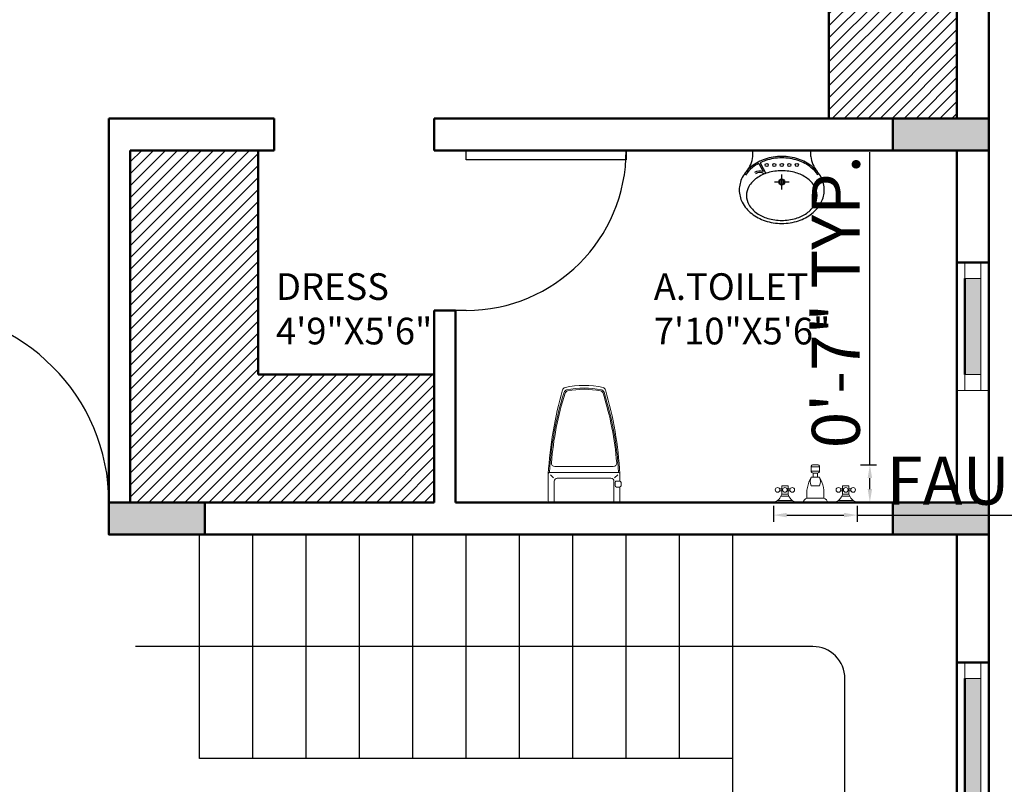
# Model space of a CAD drawing. Units: inches. Extents: x 3064 to 19385, y 846 to 15425.
# Tile 19 of 108: x 3808 to 3992, y 1134 to 1277. Entities that reach past the tile are written whole.
import ezdxf

# ---------------------------------------------------------------- set-up
doc = ezdxf.new("R2010")
doc.units = ezdxf.units.IN
for name, color, linetype, lineweight in [('A-ANNO-DIMS', 2, 'Continuous', 18), ('A-AREA-IDEN', 3, 'Continuous', 18), ('A-COLS', 1, 'Continuous', 35), ('A-DOOR', 3, 'Continuous', 25), ('A-FLOR-FIXT', 9, 'Continuous', 18), ('A-FLOR-STRS', 2, 'Continuous', 25), ('A-FURN-PATT', 252, 'Continuous', 13), ('A-GLAZ', 4, 'Continuous', 18), ('A-WALL', 7, 'Continuous', 50)]:
    doc.layers.add(name, color=color, linetype=linetype, lineweight=lineweight)
doc.layers.add('THIET-BI', color=21, linetype='Continuous')
doc.styles.get("Standard").update_dxf_attribs({"font": 'arial.ttf'})
doc.dimstyles.new('ISO-25', dxfattribs={"dimtxt": 9, "dimasz": 2.5, "dimexe": 1.25, "dimexo": 0.625, "dimtad": 1, "dimdec": 1, "dimlunit": 3, "dimtxsty": 'Standard', "dimcen": 2.5, "dimadec": 0, "dimazin": 0, "dimtfac": 1, "dimtdec": 1, "dimtmove": 0, "dimatfit": 3, "dimfxl": 1, "dimarcsym": 0})
pattern_1 = [(45, (-695.1336, 0), (-1.122532, 1.122532), [])]

# ---------------------------------------------------------------- blocks, each defined once
blk = doc.blocks.new('*U3')
for p, q in [((0, 0), (0, -6)), ((36, 0), (36, -6))]:
    blk.add_line(p, q)
blk.add_lwpolyline([(0, 0), (0, 36), (1.75, 36), (1.75, 0)], close=True)
blk.add_arc((0, 0), 36, 0, 90)
blk = doc.blocks.new('*U4')
for p, q in [((0, 0), (0, -6)), ((30, 0), (30, -6))]:
    blk.add_line(p, q)
blk.add_lwpolyline([(0, 0), (0, 30), (1.75, 30), (1.75, 0)], close=True)
blk.add_arc((0, 0), 30, 0, 90)
blk = doc.blocks.new('A$C430D11A0')
at = {"layer": 'THIET-BI'}
for p, q in [((90, 445), (90, 485)), ((475, 485), (90, 485)), ((475, 483), (90, 483)), ((475, 445), (475, 485)), ((129.4, 398.5), (158.2, 344.4)), ((138.3, 403), (176, 332.4)), ((233.4, 275.5), (331.9, 275.5)), ((282.5, 226.2), (282.5, 324.8))]:
    blk.add_line(p, q, dxfattribs=at)
for points in [[(565, 222.5, 0.121635), (544.7, 304.8, 0.10526), (482.3, 379.8, 0.088175), (393.4, 427.4, 0.079002), (282.5, 445, 0.079002), (171.6, 427.4, 0.088175), (82.7, 379.8, 0.10526), (20.3, 304.8, 0.121635), (0, 222.5, 0.121635), (20.3, 140.2, 0.10526), (82.7, 65.2, 0.088175), (171.6, 17.6, 0.079002), (282.5, 0, 0.079002), (393.4, 17.6, 0.088175), (482.3, 65.2, 0.10526), (544.7, 140.2, 0.121635)], [(517.5, 185, 0.134042), (501.2, 244.9, 0.106817), (448.7, 301.7, 0.082468), (375.6, 336.7, 0.070874), (282.5, 350, 0.070874), (189.4, 336.7, 0.082468), (116.3, 301.7, 0.106817), (63.8, 244.9, 0.134042), (47.5, 185, 0.134042), (63.8, 125.1, 0.106817), (116.3, 68.3, 0.082468), (189.4, 33.3, 0.070874), (282.5, 20, 0.070874), (375.6, 33.3, 0.082468), (448.7, 68.3, 0.106817), (501.2, 125.1, 0.134042)]]:
    blk.add_lwpolyline(points, format="xyb", close=True, dxfattribs=at)
for points in [[(129.4, 398.5, 0.043566), (88.9, 372, 0.07708), (42.1, 321.6, 0.041486)], [(522.9, 321.6, 0.07708), (476.1, 372, 0.088175), (390.3, 417.9, 0.079002), (282.5, 435, 0.079002), (174.7, 417.9, 0.035427), (138.3, 403, 0.07708)]]:
    blk.add_lwpolyline(points, format="xyb", dxfattribs=at)
for centre, radius in [((182.5, 388.2), 10.5), ((232.5, 388.2), 10.5), ((282.5, 388.2), 10.5), ((332.5, 388.2), 10.5), ((382.5, 388.2), 10.5), ((282.5, 275.5), 20), ((282.5, 275.5), 15)]:
    blk.add_circle(centre, radius, dxfattribs=at)
for centre, radius, start, end in [((-103.8, 468.9), 195.3, 320.8253, 352.95569), ((668.8, 468.9), 195.3, 187.04431, 219.1747), ((136.4, 285.4), 62.9, 69.64296, 123.47738), ((136.4, 285.4), 52.9, 55.24551, 123.47738)]:
    blk.add_arc(centre, radius, start, end, dxfattribs=at)
blk = doc.blocks.new('WC-P05')
for p, q in [((-202.4, 531.6), (-202.4, 439.1)), ((-192.4, 541.6), (262.6, 541.6)), ((-163.4, 541.6), (-163.4, 400.6)), ((233.6, 541.6), (233.6, 400.6)), ((272.6, 531.6), (272.6, 351.6)), ((-210.4, 430.1), (-210.4, 409.1)), ((-202.4, 400.1), (-202.4, 351.6)), ((-201.4, 439.1), (-180.4, 439.1)), ((-201.4, 400.1), (-180.4, 400.1)), ((-171.4, 430.1), (-171.4, 409.1)), ((-192.4, 341.6), (262.6, 341.6)), ((-166.9, 378.6), (-188.2, 357.3)), ((-143.4, 380.6), (213.6, 380.6)), ((237.1, 378.6), (258.4, 357.3)), ((-159.3, 302.6), (229.5, 302.6))]:
    blk.add_line(p, q)
blk.add_lwpolyline([(-90.9, -221.9, 0.114547), (161, -222, 0.114547)], format="xyb")
for centre, radius, start, end in [((-192.4, 531.6), 10, 90, 180), ((262.6, 531.6), 10, 0, 90), ((-201.4, 430.1), 9, 90, 180), ((-201.4, 409.1), 9, 180, 270), ((-180.4, 430.1), 9, 0, 90), ((-180.4, 409.1), 9, 270, 0), ((-143.4, 400.6), 20, 180, 270), ((213.6, 400.6), 20, 270, 0), ((2308.9, 492.3), 2515.2, 183.20675, 196.12415), ((-192.4, 351.6), 10, 180, 270), ((1906, 447.2), 2102.6, 182.87428, 197.65536), ((-1835.8, 447.2), 2102.6, 342.34464, 357.12572), ((-2238.7, 492.3), 2515.2, 343.87268, 356.79325), ((262.6, 351.6), 10, 270, 0), ((-159.3, 280.1), 22.5, 90, 184.62462), ((1905.9, 447.2), 2094.5, 184.62454, 197.52765), ((-1835.8, 447.2), 2094.6, 342.46396, 355.37538), ((229.5, 280.1), 22.5, 355.37538, 90), ((-76.1, -183.7), 22.5, 197.65536, 257.50587), ((-69.9, -176.8), 22.5, 197.52765, 258.10049), ((139.9, -177.1), 22.5, 281.73735, 342.46396), ((146.2, -183.7), 22.5, 282.49413, 342.34464), ((-85.8, -199.9), 22.5, 196.12415, 256.89941), ((35.1, 318), 536.4, 257.50587, 282.49413), ((35.7, 324.3), 534.7, 258.10049, 281.73735), ((155.9, -200.1), 22.5, 283.03778, 343.87268)]:
    blk.add_arc(centre, radius, start, end)
blk = doc.blocks.new('Faucet - Bathroom front')
for p, q in [((-0.5, 4.25), (0.5, 4.25)), ((0.5, 3.75), (-0.5, 3.75)), ((-0.5, 3), (0.5, 3)), ((-0.25, 3), (-0.25, 3.5)), ((0.25, 3.5), (0.25, 3)), ((-4, 1.625), (-4.25, 1.625)), ((-4, 1.375), (-4.25, 1.375)), ((-3.25, 1.625), (-3, 1.625)), ((-3.25, 1.375), (-3, 1.375)), ((0.5, 2), (-0.5, 2)), ((3.25, 1.625), (3, 1.625)), ((3.25, 1.375), (3, 1.375)), ((4, 1.625), (4.25, 1.625)), ((4, 1.375), (4.25, 1.375)), ((-5, 0), (-2.25, 0)), ((-4.5087, 0.25), (-2.7408, 0.25)), ((-3.1442, 0.75), (-4.0979, 0.75)), ((-1.5, 0), (1.5, 0)), ((-1, 0.5), (1, 0.5)), ((2.25, 0), (5, 0)), ((2.7413, 0.25), (4.5092, 0.25)), ((4.1058, 0.75), (3.1521, 0.75))]:
    blk.add_line(p, q)
for points in [[(-0.5, 3.75), (-0.5, 4.25)], [(-0.25, 4.5), (0.25, 4.5)], [(0.5, 4.25), (0.5, 3.75)], [(0.25, 3.5), (-0.25, 3.5)]]:
    blk.add_lwpolyline(points)
for points in [[(-4, 1), (-4, 2), (-3.25, 2), (-3.25, 1)], [(3.25, 1), (3.25, 2), (4, 2), (4, 1)]]:
    blk.add_lwpolyline(points, close=True)
for centre in [(-4.5, 1.5), (-3.625, 1.5), (-2.75, 1.5), (2.75, 1.5), (3.625, 1.5), (4.5, 1.5)]:
    blk.add_circle(centre, 0.2795)
for centre, radius, start, end in [((-0.2575, 4.2575), 0.2426, 88.22243, 181.7776), ((-0.2575, 3.7425), 0.2426, 178.2224, 271.7776), ((0.2575, 4.2575), 0.2426, 358.2224, 91.77757), ((0.2575, 3.7425), 0.2426, 268.2224, 1.777565), ((3, 1), 4.0311, 150.2551, 187.125), ((0.6413, 2.5), 1.246, 156.3417, 203.6583), ((-3, 1), 4.0311, 352.875, 29.74488), ((-0.6413, 2.5), 1.246, 336.3417, 23.65835), ((-5.375, 1.375), 1.4252, 285.2551, 344.7449), ((-1.875, 1.375), 1.4252, 195.2551, 254.7449), ((-0.7962, -0.2038), 0.7327, 106.1502, 163.8498), ((0.7962, -0.2038), 0.7327, 16.1502, 73.84979), ((1.875, 1.375), 1.4252, 285.2551, 344.7449), ((5.375, 1.375), 1.4252, 195.2551, 254.7449)]:
    blk.add_arc(centre, radius, start, end)
blk = doc.blocks.new('WIN-600')
h = blk.add_hatch(color=256)
h.dxf.hatch_style = 1
h.paths.add_polyline_path([(3, 18), (0, 18), (0, 0), (3, 0)])
blk.add_line((3, 18), (3, 0))
blk.add_lwpolyline([(3, 18), (0, 18), (0, 21), (3, 21)], close=True)
blk = doc.blocks.new('WIN-1800-PAIR')
h = blk.add_hatch(color=256)
h.dxf.hatch_style = 1
h.paths.add_polyline_path([(0, 0), (3, 0), (3, 70.5), (0, 70.5)])
h.paths.add_polyline_path([(3, 144), (0, 144), (0, 73.5), (3, 73.5)])
blk.add_line((3, 144), (3, 73.5))
blk.add_lwpolyline([(3, 144), (0, 144), (0, 147), (3, 147)], close=True)
blk = doc.blocks.new('*D407')
at = {"layer": 'A-ANNO-DIMS', "color": 0, "lineweight": -2, "transparency": 16777216}
for p, q in [((3948.96, 1185.71), (3948.96, 1182.73)), ((3964.69, 1185.71), (3964.69, 1182.73)), ((3951.46, 1183.98), (3962.19, 1183.98)), ((3964.69, 1183.98), (4097.55, 1183.98))]:
    blk.add_line(p, q, dxfattribs=at)
at = {"layer": 'A-ANNO-DIMS', "color": 0, "transparency": 16777216}
for points in [[(3951.46, 1184.4), (3951.46, 1183.56), (3948.96, 1183.98)], [(3962.19, 1184.4), (3962.19, 1183.56), (3964.69, 1183.98)]]:
    blk.add_solid(points, dxfattribs=at)
at = {"layer": 'Defpoints', "color": 0, "transparency": 16777216}
for p in [(3948.96, 1186.34), (3964.69, 1186.34), (3964.69, 1183.98)]:
    blk.add_point(p, dxfattribs=at)
at = {"layer": 'A-ANNO-DIMS', "color": 0, "transparency": 16777216, "insert": (4032.37, 1189.26), "char_height": 9, "attachment_point": 5}
blk.add_mtext('FAUCET 1\'-3 1/2" TYP.', dxfattribs=at)
blk = doc.blocks.new('*D408')
at = {"layer": 'A-ANNO-DIMS', "color": 0, "lineweight": -2, "transparency": 16777216}
for p, q in [((3967.05, 1193.42), (3967.05, 1252.03)), ((3965.32, 1193.42), (3968.3, 1193.42)), ((3967.05, 1188.84), (3967.05, 1190.92)), ((3965.32, 1186.34), (3968.3, 1186.34))]:
    blk.add_line(p, q, dxfattribs=at)
at = {"layer": 'A-ANNO-DIMS', "color": 0, "transparency": 16777216}
for points in [[(3966.64, 1190.92), (3967.47, 1190.92), (3967.05, 1193.42)], [(3966.64, 1188.84), (3967.47, 1188.84), (3967.05, 1186.34)]]:
    blk.add_solid(points, dxfattribs=at)
at = {"layer": 'Defpoints', "color": 0, "transparency": 16777216}
for p in [(3964.69, 1193.42), (3967.05, 1193.42), (3964.69, 1186.34)]:
    blk.add_point(p, dxfattribs=at)
at = {"layer": 'A-ANNO-DIMS', "color": 0, "transparency": 16777216, "insert": (3961.83, 1223.98), "char_height": 9, "attachment_point": 5, "rotation": 90}
blk.add_mtext('0\'-7" TYP.', dxfattribs=at)

msp = doc.modelspace()

# ---------------------------------------------------------------- hatches: boundary and pattern name
at = {"layer": 'A-COLS'}
h = msp.add_hatch(color=256, dxfattribs=at)
h.dxf.hatch_style = 1
h.paths.add_polyline_path([(3989.36, 1252.34), (3989.36, 1258.34), (3971.36, 1258.34), (3971.36, 1252.34)])
h = msp.add_hatch(color=256, dxfattribs=at)
h.dxf.hatch_style = 1
h.paths.add_polyline_path([(3842.36, 1180.34), (3842.36, 1186.34), (3824.36, 1186.34), (3824.36, 1180.34)])
h = msp.add_hatch(color=256, dxfattribs=at)
h.dxf.hatch_style = 1
h.paths.add_polyline_path([(3989.36, 1180.34), (3989.36, 1186.34), (3971.36, 1186.34), (3971.36, 1180.34)])
at = {"layer": 'A-FURN-PATT'}
h = msp.add_hatch(dxfattribs=at)
h.set_pattern_fill('ANSI31', color=256, scale=0.5)
h.set_pattern_definition(pattern_1)
h.paths.add_polyline_path([(3959.36, 1258.34), (3983.36, 1258.34), (3983.36, 1390.34), (3959.36, 1390.34)])
h = msp.add_hatch(dxfattribs=at)
h.set_pattern_fill('ANSI31', color=256, scale=0.5)
h.set_pattern_definition(pattern_1)
h.paths.add_polyline_path([(3852.36, 1210.34), (3852.36, 1252.34), (3828.36, 1252.34), (3828.36, 1186.34), (3842.36, 1186.34), (3885.36, 1186.34), (3885.36, 1210.34)])

# ---------------------------------------------------------------- linework, layer by layer
at = {"layer": 'A-FLOR-STRS'}
for p, q in [((3841.36, 1138.34), (3841.36, 1180.34)), ((3851.36, 1138.34), (3851.36, 1180.34)), ((3861.36, 1138.34), (3861.36, 1180.34)), ((3871.36, 1138.34), (3871.36, 1180.34)), ((3881.36, 1138.34), (3881.36, 1180.34)), ((3891.36, 1138.34), (3891.36, 1180.34)), ((3901.36, 1138.34), (3901.36, 1180.34)), ((3911.36, 1138.34), (3911.36, 1180.34)), ((3921.36, 1138.34), (3921.36, 1180.34)), ((3931.36, 1138.34), (3931.36, 1180.34)), ((3941.36, 1024.34), (3941.36, 1180.34)), ((3941.36, 1138.34), (3841.36, 1138.34))]:
    msp.add_line(p, q, dxfattribs=at)
msp.add_lwpolyline([(3848.85, 1003.34), (3956.36, 1003.34, 0.414214), (3962.36, 1009.34), (3962.36, 1153.34, 0.414214), (3956.36, 1159.34), (3829.36, 1159.34)], format="xyb", dxfattribs=at)
at = {"layer": 'A-GLAZ'}
msp.add_line((3983.36, 1207.34), (3989.36, 1207.34), dxfattribs=at)
msp.add_lwpolyline([(3987.86, 1207.34), (3984.86, 1207.34), (3984.86, 1210.34), (3987.86, 1210.34)], close=True, dxfattribs=at)
at = {"layer": 'A-WALL'}
for p, q in [((3989.36, 904.34), (3989.36, 1396.34)), ((3959.36, 1258.34), (3959.36, 1390.34)), ((3983.36, 1258.34), (3983.36, 1390.34)), ((3824.36, 1258.34), (3824.36, 1180.34)), ((3855.36, 1258.34), (3824.36, 1258.34)), ((3855.36, 1258.34), (3855.36, 1252.34)), ((3983.36, 1258.34), (3885.36, 1258.34)), ((3885.36, 1258.34), (3885.36, 1252.34)), ((3855.36, 1252.34), (3828.36, 1252.34)), ((3828.36, 1252.34), (3828.36, 1186.34)), ((3852.36, 1252.34), (3852.36, 1210.34)), ((3983.36, 1252.34), (3885.36, 1252.34)), ((3983.36, 1186.34), (3983.36, 1252.34)), ((3983.36, 1231.34), (3989.36, 1231.34)), ((3984.86, 1228.34), (3984.86, 1210.34)), ((3889.36, 1222.34), (3885.36, 1222.34)), ((3885.36, 1222.34), (3885.36, 1186.34)), ((3889.36, 1186.34), (3889.36, 1222.34)), ((3885.36, 1210.34), (3852.36, 1210.34)), ((3885.36, 1186.34), (3828.36, 1186.34)), ((3983.36, 1186.34), (3889.36, 1186.34)), ((3983.36, 1180.34), (3824.36, 1180.34)), ((3983.36, 982.34), (3983.36, 1180.34)), ((3989.36, 1156.34), (3983.36, 1156.34)), ((3984.86, 1153.34), (3984.86, 1082.84))]:
    msp.add_line(p, q, dxfattribs=at)
for points in [[(3989.36, 1258.34), (3971.36, 1258.34), (3971.36, 1252.34), (3989.36, 1252.34)], [(3842.36, 1186.34), (3824.36, 1186.34), (3824.36, 1180.34), (3842.36, 1180.34)], [(3989.36, 1186.34), (3971.36, 1186.34), (3971.36, 1180.34), (3989.36, 1180.34)]]:
    msp.add_lwpolyline(points, close=True, dxfattribs=at)

# ---------------------------------------------------------------- block references
at = {"layer": 'A-DOOR', "rotation": 270}
msp.add_blockref('*U4', (3891.36, 1252.34), dxfattribs=at)
at = {"layer": 'A-DOOR'}
msp.add_blockref('*U3', (3788.36, 1186.34), dxfattribs=at)
at = {"layer": 'A-FLOR-FIXT'}
for name, p, xscale, yscale, zscale in [('A$C430D11A0', (3942.56, 1238.65), 0.0282220760332506, 0.0282220760332506, 0.0282220760332506), ('Faucet - Bathroom front', (3956.83, 1186.34), 1.573166238287219, 1.573166238287219, 1.573166238287219)]:
    msp.add_blockref(name, p, dxfattribs=dict(at, xscale=xscale, yscale=yscale, zscale=zscale))
at = {"layer": 'A-FLOR-FIXT', "xscale": 0.0282220760332506, "yscale": 0.0282220760332506, "zscale": 0.0282220760332506, "rotation": 180}
msp.add_blockref('WC-P05', (3914.45, 1201.63), dxfattribs=at)
at = {"layer": 'A-GLAZ'}
for name, p in [('WIN-600', (3984.86, 1210.34)), ('WIN-1800-PAIR', (3984.86, 1009.34))]:
    msp.add_blockref(name, p, dxfattribs=at)

# ---------------------------------------------------------------- texts
at = {"layer": 'A-AREA-IDEN', "char_height": 5, "attachment_point": 1}
for s, insert in [('DRESS\\P4\'9"X5\'6"', (3855.69, 1229.31)), ('A.TOILET\\P7\'10"X5\'6"', (3926.53, 1229.31))]:
    msp.add_mtext_dynamic_manual_height_columns(s, width=67.5924, gutter_width=12.5, heights=[0], dxfattribs=dict(at, insert=insert))

# ---------------------------------------------------------------- dimensions: what is measured, and where the dimension line sits
at = {"layer": 'A-ANNO-DIMS'}
dim = msp.add_linear_dim(base=(3967.05, 1193.42), p1=(3964.69, 1186.34), p2=(3964.69, 1193.42), angle=90, text='<> TYP.', dimstyle='ISO-25', override={"dimdec": 1, "dimrnd": 0, "dimzin": 1, "dimlunit": 4, "dimfrac": 2}, dxfattribs=at)
dim.commit()
dim.dimension.update_dxf_attribs({"geometry": '*D408', "text_midpoint": (3961.83, 1223.98)})
dim = msp.add_linear_dim(base=(3964.69, 1183.98), p1=(3948.96, 1186.34), p2=(3964.69, 1186.34), text='FAUCET <> TYP.', dimstyle='ISO-25', override={"dimdec": 1, "dimrnd": 0, "dimzin": 1, "dimlunit": 4, "dimfrac": 2}, dxfattribs=at)
dim.commit()
dim.dimension.update_dxf_attribs({"geometry": '*D407', "text_midpoint": (4032.37, 1189.26)})

doc.saveas('drawing.dxf')
